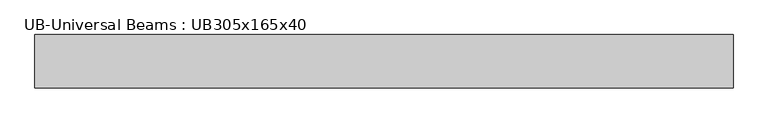
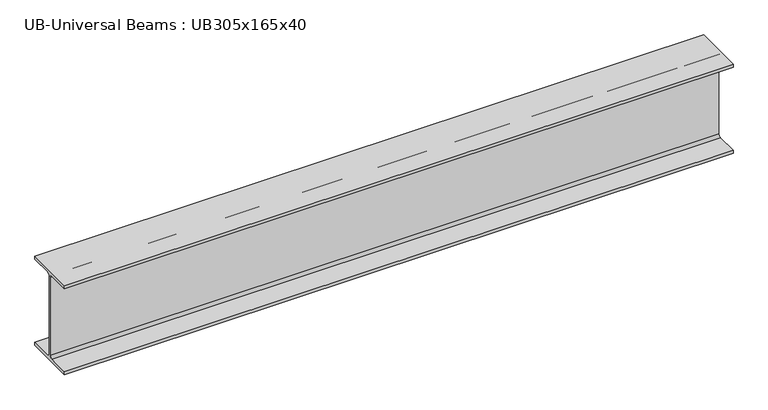
"""IFC4 building model written with IfcOpenShell, lengths in millimetres: beam geometry, UB-Universal Beams : UB305x165x40."""

from ifc_helpers import new_model, si_unit, point, frame, frame_2d, origin, place, context, project, spatial, polyline, circle_curve, trimmed, segment, composite_curve, outline, extrude, source, transform, mapped, element, save


def ub_universal_beams_ub305x165x40_0b6a72e4(model_context):
    return source(origin(), model_context, "Body", "SweptSolid", [
        extrude(outline(composite_curve([segment(polyline([(82.5, -141.5), (82.5, -151.7), (-82.5, -151.7), (-82.5, -141.5), (-11.9, -141.5)]), True, "CONTINUOUS"), segment(trimmed(circle_curve(frame_2d((-11.9, -132.6)), 8.9), [point((-11.9, -141.5))], [point((-3.0, -132.6))], True, "CARTESIAN"), True, "CONTINUOUS"), segment(polyline([(-3.0, -132.6), (-3.0, 132.6)]), True, "CONTINUOUS"), segment(trimmed(circle_curve(frame_2d((-11.9, 132.6)), 8.9), [point((-3.0, 132.6))], [point((-11.9, 141.5))], True, "CARTESIAN"), True, "CONTINUOUS"), segment(polyline([(-11.9, 141.5), (-82.5, 141.5), (-82.5, 151.7), (82.5, 151.7), (82.5, 141.5), (11.9, 141.5)]), True, "CONTINUOUS"), segment(trimmed(circle_curve(frame_2d((11.9, 132.6)), 8.9), [point((11.9, 141.5))], [point((3.0, 132.6))], True, "CARTESIAN"), True, "CONTINUOUS"), segment(polyline([(3.0, 132.6), (3.0, -132.6)]), True, "CONTINUOUS"), segment(trimmed(circle_curve(frame_2d((11.9, -132.6)), 8.9), [point((3.0, -132.6))], [point((11.9, -141.5))], True, "CARTESIAN"), True, "CONTINUOUS"), segment(polyline([(11.9, -141.5), (82.5, -141.5)]), True, "CONTINUOUS")], self_intersect=False)), frame((-588.8, 0.0, 0.0), z_axis=(1.0, 0.0, 0.0), x_axis=(0.0, 1.0, 0.0)), (0.0, 0.0, 1.0), 2152.8),
    ])


if __name__ == "__main__":
    model = new_model("IFC4")
    model_context = context("Model", 3, world=origin())
    ifc_project = project(units=[si_unit("LENGTHUNIT", "METRE", prefix="MILLI")], contexts=[model_context])
    site = spatial("IfcSite", under=ifc_project)
    building = spatial("IfcBuilding", under=site)
    placement = place(None, origin())
    ub_universal_beams_ub305x165x40_shape = ub_universal_beams_ub305x165x40_0b6a72e4(model_context)
    element("IfcBeam", 1, ObjectType="UB-Universal Beams : UB305x165x40", at=placement, inside=building, context=model_context, shape_type="MappedRepresentation", body=[
        mapped(ub_universal_beams_ub305x165x40_shape, transform((0.0, 0.0, 0.0), x_axis=(1.0, 0.0, 0.0), y_axis=(0.0, 1.0, 0.0), z_axis=(0.0, 0.0, 1.0))),
    ])
    save(model, "model.ifc")

# Revit data of these elements
# Type "UB-Universal Beams : UB305x165x40"
#   Section Name Key = "UB305X165X40"
#   Width = 16.5 cm
#   Web Thickness = 0.6 cm
#   Web Fillet = 0.89 cm
#   Warping Constant = 164000.0 cm⁶
#   Torsional Moment of Inertia = 14.70 cm⁴
#   Section Area = 51.3 cm²
#   Plastic Modulus weak axis = 142.0 cm³
#   Plastic Modulus strong axis = 623.0 cm³
#   Nominal Weight = 40.2999 kgf/m
#   Moment of Inertia weak axis = 764.00 cm⁴
#   Moment of Inertia strong axis = 8503.00 cm⁴
#   Height = 30.34 cm
#   Flange Thickness = 1.02 cm
#   Elastic Modulus weak axis = 92.6 cm³
#   Elastic Modulus strong axis = 560.0 cm³
#   Centroid Vertical = 15.17 cm
#   Centroid Horizontal = 8.25 cm
#   Bolt Spacing = 9.0 cm
#   Length [instance default] = 1500 mm
#   Structural Material [instance default] = Metal - Steel 43-275
#   Type Comments = ""
#   Assembly Code = ""
# Element 1 (IfcBeam, "UB-Universal Beams : UB305x165x40")
#   Materials on its faces: "Metal - Steel 43-275"
# Materials
#   "Metal - Steel 43-275": class "Metal", colour RGB 247 247 247, transparency 0, Cost = 0
